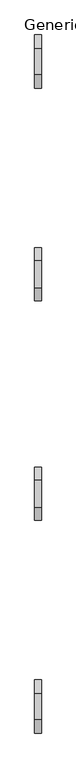
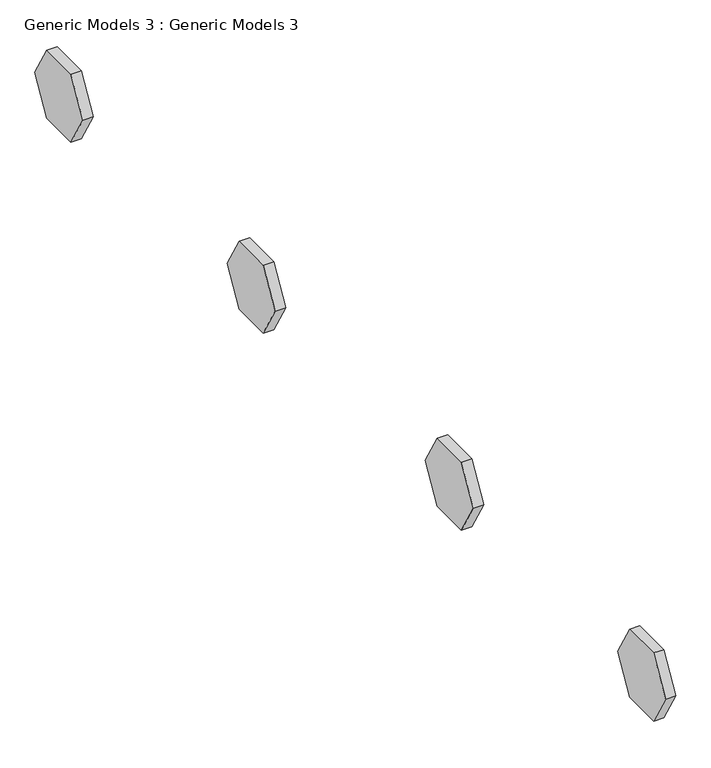
"""IFC4 building model written with IfcOpenShell, lengths in millimetres: proxy geometry, Generic Models 3 : Generic Models 3."""

from ifc_helpers import new_model, si_unit, frame, origin, place, context, project, spatial, polyline, outline, extrude, source, transform, mapped, element, save


def generic_models_3_generic_models_3_906b0088(model_context):
    return source(origin(), model_context, "Body", "SweptSolid", [
        extrude(outline(polyline([(-6567.6337185, 1279.5855827), (-6262.8337185, 751.6564966), (-6567.6337185, 223.7274104), (-7177.2337185, 223.7274104), (-7482.0337185, 751.6564966), (-7177.2337185, 1279.5855827), (-6567.6337185, 1279.5855827)])), frame((5837.7486397, 0.0, 0.0), z_axis=(1.0, 0.0, 0.0), x_axis=(0.0, 1.0, 0.0)), (0.0, 0.0, 1.0), 152.4),
        extrude(outline(polyline([(-1690.8337185, 1279.5855827), (-1386.0337185, 751.6564966), (-1690.8337185, 223.7274104), (-2300.4337185, 223.7274104), (-2605.2337185, 751.6564966), (-2300.4337185, 1279.5855827), (-1690.8337185, 1279.5855827)])), frame((5837.7486397, 0.0, 0.0), z_axis=(1.0, 0.0, 0.0), x_axis=(0.0, 1.0, 0.0)), (0.0, 0.0, 1.0), 152.4),
        extrude(outline(polyline([(3338.3662815, 1279.5855827), (3643.1662815, 751.6564966), (3338.3662815, 223.7274104), (2728.7662815, 223.7274104), (2423.9662815, 751.6564966), (2728.7662815, 1279.5855827), (3338.3662815, 1279.5855827)])), frame((5837.7486397, 0.0, 0.0), z_axis=(1.0, 0.0, 0.0), x_axis=(0.0, 1.0, 0.0)), (0.0, 0.0, 1.0), 152.4),
        extrude(outline(polyline([(8215.1662815, 1279.5855827), (8519.9662815, 751.6564966), (8215.1662815, 223.7274104), (7605.5662815, 223.7274104), (7300.7662815, 751.6564966), (7605.5662815, 1279.5855827), (8215.1662815, 1279.5855827)])), frame((5837.7486397, 0.0, 0.0), z_axis=(1.0, 0.0, 0.0), x_axis=(0.0, 1.0, 0.0)), (0.0, 0.0, 1.0), 152.4),
    ])


if __name__ == "__main__":
    model = new_model("IFC4")
    model_context = context("Model", 3, world=origin())
    ifc_project = project(units=[si_unit("LENGTHUNIT", "METRE", prefix="MILLI")], contexts=[model_context])
    site = spatial("IfcSite", under=ifc_project)
    building = spatial("IfcBuilding", under=site)
    placement = place(None, origin())
    generic_models_3_generic_models_3_shape = generic_models_3_generic_models_3_906b0088(model_context)
    element("IfcBuildingElementProxy", 1, Name="Generic Models 3 : Generic Models 3", ObjectType="Generic Models 3 : Generic Models 3", at=placement, inside=building, context=model_context, shape_type="MappedRepresentation", body=[
        mapped(generic_models_3_generic_models_3_shape, transform((0.0, 0.0, 0.0), x_axis=(1.0, 0.0, 0.0), y_axis=(0.0, 1.0, 0.0), z_axis=(0.0, 0.0, 1.0))),
    ])
    save(model, "model.ifc")

# Revit data of these elements
# Element 1 (IfcBuildingElementProxy, "Generic Models 3 : Generic Models 3")
#   Materials on its faces: "Door - Frame"
# Materials
#   "Door - Frame": colour RGB 118 70 51, transparency 0, Cost = 0
